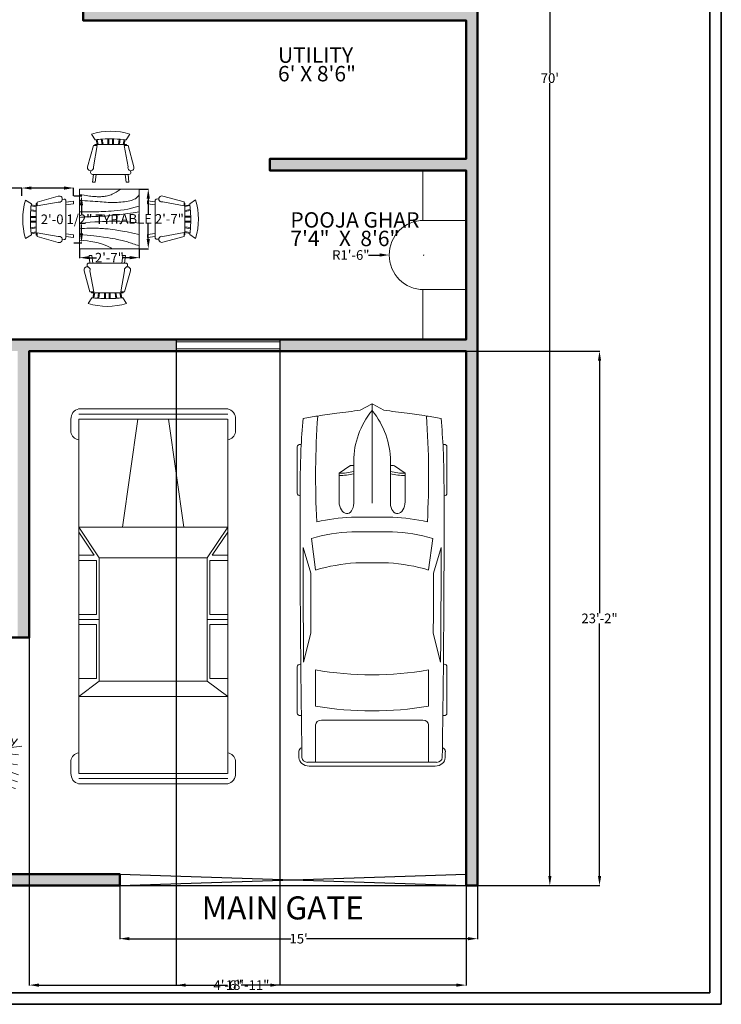
# Model space of a CAD drawing. Units: inches. Extents: x -60 to 743, y -483 to 510.
# Tile 4 of 7: x 378 to 743, y -483 to 29. Entities that reach past the tile are written whole.
import ezdxf

# ---------------------------------------------------------------- set-up
doc = ezdxf.new("R2010")
doc.units = ezdxf.units.IN
doc.header["$MEASUREMENT"] = 0
for name, color, linetype, lineweight in [('A-ANNO-DIMS', 2, 'Continuous', 18), ('A-ANNO-TEXT', 7, 'Continuous', 25), ('A-ANNO-TTLB', 7, 'Continuous', 35), ('A-AREA-IDEN', 7, 'Continuous', 25), ('A-WALL-PATT', 30, 'Continuous', 13), ('CARS', 131, 'Continuous', 13), ('FURNITURE', 40, 'Continuous', 18), ('GATE', 150, 'Continuous', 25), ('TREES', 80, 'Continuous', 13), ('WALL BOUNDRY', 10, 'Continuous', 50), ('WINDOW', 200, 'Continuous', 18)]:
    doc.layers.add(name, color=color, linetype=linetype, lineweight=lineweight)
doc.styles.get("Standard").update_dxf_attribs({"font": 'arial.ttf'})
doc.dimstyles.get("Standard").update_dxf_attribs({"dimtxt": 5, "dimasz": 5, "dimexe": 0.18, "dimexo": 0.0625, "dimgap": 0.09, "dimtad": 0, "dimtih": 1, "dimtoh": 1, "dimdec": 1, "dimzin": 0, "dimdsep": 46, "dimlunit": 4, "dimtxsty": 'Standard', "dimcen": 0.09, "dimadec": 0, "dimazin": 0, "dimtfac": 1, "dimtdec": 1, "dimtofl": 0, "dimtmove": 0, "dimatfit": 3, "dimfxl": 1, "dimtolj": 1, "dimtzin": 0, "dimarcsym": 0})

# ---------------------------------------------------------------- blocks, each defined once
blk = doc.blocks.new('Chair - Rocking')
for p, q in [((-8, -4.5), (-10, -1.5)), ((-7.5, -4.5), (-7, -7)), ((-6.5, -7), (-7.02225, -4.43)), ((-4.5, -7), (-4.96674, -4.19951)), ((-4, -7), (-4.40532, -4.16272)), ((-1.5, -4.05012), (-1.5, -7)), ((-1, -7), (-1, -4.05012)), ((1, -7), (1, -4.04655)), ((1.5, -4.05012), (1.5, -7)), ((4, -7), (4.40187, -4.18694)), ((4.5, -7), (4.96761, -4.19437)), ((6.5, -7), (7, -4.4057)), ((7.5, -4.5), (7, -7)), ((8, -4.5), (10, -1.5)), ((-9, -7.5), (-12, -18.49999)), ((-7, -7.5), (-9, -7.5)), ((-9, -18.49999), (-7, -7.5)), ((-8.23428, -6.99939), (-8.3093, -7.47958)), ((-8.23041, -7), (8.23915, -7)), ((7, -7.5), (9, -7.5)), ((9, -18.49999), (7, -7.5)), ((8.31071, -7.48854), (8.23449, -7.00073)), ((9, -7.5), (12, -18.49999)), ((-10.36644, -20.64523), (-10.5, -21.49999)), ((-9, -22.49999), (-9.5, -26.49999)), ((0, -22.49999), (-9.5, -22.49999)), ((-8, -26.49999), (-7.5, -22.49999)), ((0, -22.49999), (9.5, -22.49999)), ((8, -26.49999), (7.5, -22.49999)), ((9, -22.49999), (9.5, -26.49999)), ((10.5, -21.49999), (10.3575, -20.58798)), ((-9.5, -26.49999), (-8, -26.49999)), ((9.5, -26.49999), (8, -26.49999))]:
    blk.add_line(p, q)
for centre, radius, start, end in [((0, -34.08333), 34.08333, 72.93847, 107.0615), ((0, -68.25004), 64.25, 93.92211, 97.15267), ((0, -68.25004), 64.25, 82.84733, 93.92211), ((-10.5, -18.99999), 1.58114, 161.5651, 18.43495), ((10.5, -18.99999), 1.58114, 161.5651, 18.43495), ((-9.5, -21.49999), 1, 180, 270), ((9.5, -21.49999), 1, 270, 0)]:
    blk.add_arc(centre, radius, start, end)
blk = doc.blocks.new('Table - Square Woodgrain 42 x 42 in.')
blk.add_line((0, -42), (42, -42))
for points in [[(0, -4), (1.704, -4.2172), (3.2358, -4.4188), (4.615, -4.604), (5.8615, -4.7721), (6.9951, -4.9224), (8.0357, -5.0541), (9.0031, -5.1667), (9.9171, -5.2594), (10.7951, -5.3316), (11.6445, -5.3836), (12.4702, -5.4157), (13.277, -5.4283), (14.0698, -5.4217), (14.8535, -5.3964), (15.6331, -5.3526), (16.4133, -5.2908), (17.1986, -5.2103), (17.9913, -5.1062), (18.793, -4.9727), (19.6056, -4.8038), (20.4307, -4.5937), (21.2701, -4.3365), (22.1256, -4.0262), (22.9989, -3.6571), (23.888, -3.2272), (24.7756, -2.7516), (25.6408, -2.2491), (26.4624, -1.7387), (27.2195, -1.2395), (27.891, -0.7703), (28.456, -0.3501), (28.8934, 0.002)], [(0, -42), (0, 0), (42, 0), (42, -42)], [(0, -8), (1.8203, -8.1001), (3.6741, -8.2149), (5.5411, -8.3408), (7.4011, -8.4741), (9.2339, -8.6112), (11.0193, -8.7484), (12.7371, -8.8821), (14.3671, -9.0086), (15.8954, -9.1246), (17.3337, -9.2278), (18.6997, -9.3159), (20.0116, -9.387), (21.2871, -9.4389), (22.5442, -9.4696), (23.8008, -9.477), (25.0749, -9.459), (26.3791, -9.4137), (27.7049, -9.3403), (29.0383, -9.2382), (30.3655, -9.1068), (31.6728, -8.9455), (32.9461, -8.7535), (34.1717, -8.5304), (35.3358, -8.2756), (36.4268, -7.9863), (37.443, -7.6521), (38.3849, -7.2603), (39.253, -6.7986), (40.048, -6.2542), (40.7705, -5.6147), (41.421, -4.8674), (42, -4)], [(42, -12), (39.1784, -12.8621), (36.4519, -13.5654), (33.8246, -14.1294), (31.3004, -14.5731), (28.8832, -14.9161), (26.577, -15.1775), (24.3858, -15.3768), (22.3136, -15.5332), (20.3622, -15.6632), (18.5254, -15.7718), (16.7947, -15.8612), (15.1618, -15.9338), (13.6183, -15.9916), (12.1558, -16.0369), (10.7659, -16.0718), (9.4403, -16.0987), (8.1703, -16.1191), (6.9461, -16.1325), (5.7577, -16.1377), (4.595, -16.1335), (3.4479, -16.1188), (2.3064, -16.0924), (1.1604, -16.0532), (0, -16)], [(42, -16), (37.6529, -16.7365), (33.8802, -17.329), (30.6179, -17.7961), (27.8015, -18.1561), (25.3668, -18.4275), (23.2497, -18.6288), (21.3859, -18.7785), (19.7111, -18.8949), (18.1693, -18.9939), (16.7375, -19.0795), (15.401, -19.1534), (14.1449, -19.217), (12.9544, -19.2717), (11.8148, -19.3191), (10.7113, -19.3606), (9.6291, -19.3976), (8.5534, -19.4323), (7.47, -19.4689), (6.3643, -19.5122), (5.222, -19.5672), (4.0288, -19.6386), (2.7703, -19.7313), (1.4321, -19.8501), (0, -20)], [(0, -24), (3.9243, -23.6805), (7.4766, -23.4138), (10.6891, -23.1954), (13.5943, -23.0205), (16.2247, -22.8847), (18.6125, -22.7832), (20.7903, -22.7116), (22.7903, -22.6651), (24.6563, -22.642), (26.4764, -22.6507), (28.35, -22.7024), (30.3766, -22.8084), (32.6555, -22.98), (35.2861, -23.2283), (38.3678, -23.5645), (42, -24)], [(42, -32), (37.392, -31.017), (33.4585, -30.2231), (30.1291, -29.5949), (27.3334, -29.109), (25.0009, -28.742), (23.0612, -28.4707), (21.4439, -28.2716), (20.0786, -28.1215), (18.8998, -28.0002), (17.8609, -27.9014), (16.9206, -27.8219), (16.0371, -27.7588), (15.1691, -27.709), (14.2748, -27.6693), (13.3128, -27.6368), (12.2415, -27.6083), (11.0295, -27.5824), (9.6867, -27.5643), (8.233, -27.5608), (6.6884, -27.5787), (5.0728, -27.6248), (3.4062, -27.7058), (1.7086, -27.8286), (0, -28)], [(0, -32), (5.4026, -32.5358), (9.9494, -33.019), (13.7424, -33.4553), (16.8834, -33.8505), (19.4743, -34.2106), (21.6171, -34.5413), (23.4136, -34.8486), (24.9657, -35.1382), (26.3614, -35.4156), (27.6332, -35.6841), (28.7995, -35.9467), (29.8788, -36.2064), (30.8897, -36.4661), (31.8507, -36.7288), (32.7802, -36.9973), (33.6968, -37.2747), (34.6175, -37.5635), (35.5531, -37.8651), (36.5128, -38.1805), (37.506, -38.5108), (38.5421, -38.8568), (39.6302, -39.2197), (40.7797, -39.6004), (42, -40)], [(0, -36), (3.0098, -36.2857), (5.5354, -36.5643), (7.6368, -36.8359), (9.374, -37.1009), (10.807, -37.3597), (11.9957, -37.6126), (13.0002, -37.8599), (13.8804, -38.102), (14.6874, -38.3393), (15.4365, -38.5729), (16.1338, -38.8041), (16.7858, -39.0341), (17.3987, -39.264), (17.9787, -39.4952), (18.5322, -39.7288), (19.0655, -39.9662), (19.5832, -40.2081), (20.0842, -40.4544), (20.5657, -40.7046), (21.0249, -40.9581), (21.459, -41.2144), (21.8653, -41.4731), (22.2409, -41.7335), (22.5831, -41.9951)]]:
    blk.add_lwpolyline(points)
blk = doc.blocks.new('*U19')
for p, q in [((536, 950), (536, 936)), ((1182, 988), (568, 988)), ((1214, 950), (1214, 950)), ((2235, 810), (1899, 912)), ((3440, 942), (3440, 950)), ((3472, 988), (4087, 988)), ((4119, 950), (4119, 934)), ((1779, 801), (2195, 746)), ((3412, 904), (3030, 807)), ((4736, -851), (4736, 851)), ((4785, -832), (4785, 832)), ((3516, 746), (3994, 746)), ((4179, 670), (4179, -670)), ((4736, 746), (4242, 746)), ((820, 295), (918, 436)), ((918, 436), (1294, 436)), ((816, 241), (816, 283)), ((1496, -274), (1496, 274)), ((1690, -267), (1690, 267)), ((4736, -267), (4736, 267)), ((83, 156), (3, 10)), ((756, 241), (1313, 241)), ((2102, 216), (2102, -216)), ((0, 0), (1313, 0)), ((3, -10), (83, -156)), ((756, -241), (1313, -241)), ((816, -241), (816, -283)), ((820, -295), (918, -436)), ((918, -436), (1294, -436)), ((2195, -746), (1779, -801)), ((3994, -746), (3516, -746)), ((4242, -746), (4736, -746)), ((2235, -810), (1899, -912)), ((3412, -904), (3030, -807)), ((536, -950), (536, -936)), ((1182, -988), (568, -988)), ((1214, -950), (1214, -950)), ((3440, -942), (3440, -950)), ((3472, -988), (4087, -988)), ((4119, -950), (4119, -934))]:
    blk.add_line(p, q)
for centre, major_axis, ratio, start_param, end_param in [((6757, -699), (0, 7958), 0.842304, 1.367076, 1.39176), ((1046, -12468), (0, 13417), 0.842304, 0.00281, 0.075598), ((568, 950), (0, -37.6), 0.842304, 3.141593, 4.712389), ((1638, -268113), (0, 269063), 0.842304, -0.013397, 0.002797), ((1182, 950), (0, 37.6), 0.842304, -1.570796, 0), ((1638, -268113), (0, -269025), 0.842304, 3.133765, 3.140441), ((3472, 950), (0, -37.6), 0.842304, 3.141593, 4.712389), ((4087, 950), (0, 37.6), 0.842304, -1.570796, 0), ((4588, 910), (0, 56.4), 0.842304, -0.013017, 1.249894), ((1638, -268131), (0, 269121), 0.842304, -0.013397, -0.013017), ((4673, 851), (0, -75.2), 0.842304, 1.570796, 3.128196), ((4673, 832), (0, -133), 0.842304, 1.570796, 3.128196), ((3436, 137), (0, 2077), 0.842304, 1.245306, 1.50788), ((2433, -93125), (0, -93935), 0.842304, 3.134049, 3.144098), ((6583, -699), (0, -7755), 0.842304, 4.528606, 4.561838), ((952, -15087), (0, -15833), 0.842304, 3.096046, 3.200911), ((3414, 137), (0, -2280), 0.842304, 4.449482, 4.652344), ((3800, 71), (0, -2021), 0.842304, 4.372215, 4.640744), ((434, 0), (0, 3734), 0.842304, 4.511394, 4.913384), ((912, 0), (0, 3734), 0.842304, 4.511394, 4.913384), ((4242, 670), (0, 75.2), 0.842304, 0, 1.570796), ((-5194, 1331), (0, -6374), 0.842304, 1.385369, 1.434372), ((331, 432), (0, 696), 0.842304, 4.435146, 4.718221), ((361, 432), (0, 696), 0.842304, 4.435146, 4.718221), ((1290, 339), (161, -9), 0.603834, -1.395552, 1.581315), ((832, 283), (0, 18.8), 0.842304, 0.879714, 1.570796), ((756, -1185), (0, 1427), 0.842304, 0, 0.590319), ((16, 0), (0, -18.8), 0.842304, 4.131459, 5.293319), ((756, 1185), (0, 1427), 0.842304, 2.551274, 3.141593), ((-5194, -1331), (0, 6374), 0.842304, -1.434372, -1.385369), ((331, -432), (0, -696), 0.842304, 1.564964, 1.848039), ((361, -432), (0, -696), 0.842304, 1.564964, 1.848039), ((3800, -71), (0, -2021), 0.842304, -1.499151, -1.230623), ((832, -283), (0, -18.8), 0.842304, 4.712389, 5.403472), ((3414, -137), (0, -2280), 0.842304, -1.510751, -1.307889), ((3436, -137), (0, -2077), 0.842304, -1.50788, -1.245306), ((6583, 699), (0, 7755), 0.842304, 1.721348, 1.754579), ((6757, 699), (0, 7958), 0.842304, 1.749832, 1.774517), ((952, 15087), (0, -15833), 0.842304, -0.059319, 0.045547), ((4242, -670), (0, -75.2), 0.842304, 4.712389, 6.283185), ((1638, 268113), (0, -269025), 0.842304, 0.001152, 0.007828), ((2433, 93125), (0, -93935), 0.842304, -0.002505, 0.007544), ((4673, -851), (0, 75.2), 0.842304, 3.15499, 4.712389), ((4673, -832), (0, -133), 0.842304, 0.013397, 1.570796), ((1046, 12468), (0, -13417), 0.842304, -0.075598, -0.00281), ((568, -950), (0, 37.6), 0.842304, 1.570796, 3.141593), ((1638, 268113), (0, 269063), 0.842304, 3.138796, 3.15499), ((1182, -950), (0, -37.6), 0.842304, 0, 1.570796), ((3472, -950), (0, -37.6), 0.842304, -1.570796, 0), ((4087, -950), (0, 37.6), 0.842304, 3.141593, 4.712389), ((4588, -910), (0, -56.4), 0.842304, -1.249894, 0.013017), ((1638, 268131), (0, 269121), 0.842304, 3.15461, 3.15499)]:
    blk.add_ellipse(centre, major_axis=major_axis, ratio=ratio, start_param=start_param, end_param=end_param)
at = {"extrusion": (0, 0, -1)}
blk.add_ellipse((1290, -339), major_axis=(161, 9), ratio=0.603834, start_param=-1.395552, end_param=1.581315, dxfattribs=at)
blk = doc.blocks.new('*U18')
for p, q in [((138, 1075), (308, 1075)), ((4818, 1075), (4649, 1075)), ((3, -10), (3, 974)), ((70, -10), (70, 973)), ((138, 973), (410, 973)), ((138, -10), (138, 971)), ((410, 973), (4581, 973)), ((1563, -10), (1563, 973)), ((1563, 973), (1969, 702)), ((1630, 973), (1936, 769)), ((1936, 769), (1936, 973)), ((2003, 973), (2003, 736)), ((2716, 736), (2716, 973)), ((2783, 702), (2783, 973)), ((2851, 973), (2851, 736)), ((3563, 736), (3563, 973)), ((3597, 702), (3801, 973)), ((3801, -10), (3801, 973)), ((4818, 973), (4547, 973)), ((4818, -10), (4818, 971)), ((4886, -10), (4886, 973)), ((4954, -10), (4954, 974)), ((1969, 702), (3597, 702)), ((1969, -10), (1969, 702)), ((2003, 736), (2716, 736)), ((2851, 736), (3563, 736)), ((3597, -10), (3597, 702)), ((138, 193), (1563, 396)), ((3, -11), (3, -995)), ((70, -10), (70, -994)), ((138, -11), (138, -992)), ((1563, -10), (1563, -994)), ((1969, -10), (1969, -723)), ((3597, -10), (3597, -723)), ((3801, -10), (3801, -994)), ((4818, -11), (4818, -992)), ((4886, -10), (4886, -994)), ((4954, -11), (4954, -995)), ((138, -214), (1563, -417)), ((1563, -994), (1969, -723)), ((1969, -723), (3597, -723)), ((2003, -994), (2003, -757)), ((2003, -757), (2716, -757)), ((2716, -757), (2716, -994)), ((2783, -723), (2783, -994)), ((2851, -757), (3563, -757)), ((2851, -994), (2851, -757)), ((3563, -757), (3563, -994)), ((3597, -723), (3801, -994)), ((1630, -994), (1936, -790)), ((1936, -790), (1936, -994)), ((138, -994), (410, -994)), ((410, -994), (4581, -994)), ((4818, -994), (4547, -994)), ((138, -1096), (308, -1096)), ((4818, -1096), (4649, -1096))]:
    blk.add_line(p, q)
for centre, radius, start, end in [((128, 946), 129, 85.6455, 168.0943), ((291, 956), 120, 8.1301, 81.87), ((4665, 956), 120, 98.13, 171.8699), ((4828, 946), 129, 11.9057, 94.3545), ((128, -967), 129, 191.9057, 274.3545), ((291, -977), 120, 278.13, 351.8699), ((4665, -977), 120, 188.1301, 261.87), ((4828, -967), 129, 265.6455, 348.0943)]:
    blk.add_arc(centre, radius, start, end)
blk = doc.blocks.new('*U21')
for p, q in [((-258.7244, 1362.456), (-332.3336, 1421.4348)), ((0, 0), (-266.7, 1447.8)), ((-231.1146, 1315.2628), (-166.7002, 1421.4348)), ((-221.9198, 1197.3052), (-433.5526, 1338.8594)), ((-194.31, 1102.9442), (-65.4812, 1256.284)), ((-148.3106, 914.1968), (118.5418, 1220.9018)), ((-185.1152, 1008.5578), (-553.1612, 1185.4942)), ((-129.8956, 701.8528), (265.7602, 1185.4942)), ((-93.091, 489.5342), (-700.3796, 902.3858)), ((-129.8956, 713.6638), (-626.7704, 1032.1544)), ((-74.7014, 418.7444), (219.7608, 961.39)), ((685.8, 228.6), (1219.2, 914.4)), ((689.0258, 230.0224), (790.2448, 914.1968)), ((983.4626, 867.0036), (1066.2666, 725.4494)), ((1121.4862, 925.9824), (1149.0706, 831.6214)), ((-1234.059, 536.7274), (-1252.4486, 737.2604)), ((-1105.2302, 725.4494), (-1077.6458, 395.1732)), ((-902.8176, 713.6638), (-617.5756, 100.2538)), ((412.9786, 147.447), (587.8068, 796.2392)), ((560.197, 182.8292), (698.2206, 819.8358)), ((808.6344, 784.4282), (827.0494, 418.7444)), ((891.4384, 831.6214), (946.658, 572.1096)), ((1112.2914, 760.8316), (1296.3144, 784.4282)), ((-800.1, 114.3), (-1333.5, 647.7)), ((-976.4268, 666.4706), (-884.4026, 194.6402)), ((-369.1382, 53.086), (-783.1836, 642.874)), ((-617.5756, 607.4918), (-74.7014, 347.98)), ((-28.6766, 171.0436), (228.9556, 678.2816)), ((100.1268, 41.275), (284.1498, 619.2774)), ((256.5654, 88.4682), (449.7832, 666.4706)), ((1029.462, 654.685), (1241.0948, 631.0884)), ((-1206.4492, 501.3198), (-1418.082, 465.9376)), ((-1031.621, 347.98), (-1399.667, 277.1902)), ((-525.5514, 347.98), (-28.6766, 123.8504)), ((845.439, 418.7444), (1241.0948, 277.1902)), ((919.0482, 501.3198), (1222.6798, 454.152)), ((0, 0), (685.8, 228.6)), ((615.4166, 194.6402), (1185.8752, 41.275)), ((753.4148, 312.5978), (1222.6798, 159.2326)), ((-847.598, 159.2326), (-1326.0578, 135.636)), ((-718.7946, 88.4682), (-1215.644, -147.447)), ((-543.9664, 76.6572), (-967.2066, -206.4512)), ((0, 0), (-800.1, 114.3)), ((-405.9428, 53.086), (-764.794, -241.8334)), ((0, 0), (-571.5, -495.3)), ((-166.7002, 29.4894), (-543.9664, -206.4512)), ((0, 0), (457.2, -571.5)), ((164.5412, 41.275), (661.416, -218.2368)), ((284.1498, 88.4682), (781.0246, -147.447)), ((458.978, 147.447), (891.4384, -88.4682)), ((-166.7002, -147.447), (-507.1618, -253.619)), ((-120.7008, -88.4682), (-93.091, -371.5766)), ((63.3222, -76.6826), (-37.8714, -513.1308)), ((44.9326, -64.897), (615.4166, -241.8334)), ((127.7366, -159.258), (54.1274, -654.685)), ((-387.5278, -324.4088), (-764.794, -324.4088)), ((-341.5284, -289.0012), (-221.9198, -831.6214)), ((-240.3094, -218.2368), (-157.5054, -595.7062)), ((228.9556, -289.0012), (90.932, -914.1968)), ((192.151, -230.0224), (817.8292, -371.5766)), ((-442.7474, -383.3876), (-1086.8406, -477.7486)), ((-571.5, -495.3), (-952.5, -1143)), ((-525.5514, -465.963), (-451.9422, -1126.5408)), ((-433.5526, -383.3876), (-323.1134, -1020.3688)), ((357.759, -430.5554), (164.5412, -1020.3688)), ((311.7596, -383.3876), (937.4378, -477.7486)), ((412.9786, -501.3452), (919.0482, -583.9206)), ((-617.5756, -548.5384), (-1077.6458, -560.324)), ((-681.9646, -666.496), (-1022.4262, -654.685)), ((-635.9652, -607.5172), (-580.771, -1150.1374)), ((458.978, -572.1096), (210.5406, -1161.923)), ((457.2, -571.5), (685.8, -1333.5)), ((468.1982, -572.1096), (1029.462, -737.2604)), ((486.5878, -642.8994), (983.4626, -843.4324)), ((-718.7946, -737.2604), (-1086.8406, -796.2392)), ((-737.1842, -784.4536), (-709.5744, -1114.7298)), ((514.1976, -772.6426), (403.7838, -1138.3264)), ((541.8074, -831.6214), (992.6574, -1032.1544)), ((-783.1836, -867.029), (-1077.6458, -902.4112)), ((-875.2078, -1008.5832), (-1040.8412, -1079.3476)), ((-829.2084, -937.7934), (-810.7934, -1126.5408)), ((578.612, -961.39), (495.7826, -1232.7128)), ((578.612, -973.1756), (873.0488, -1138.3264)), ((624.6114, -1161.923), (587.8068, -1291.6916)), ((624.6114, -1102.9442), (781.0246, -1209.1162)), ((679.8056, -1268.095), (716.6102, -1291.6916))]:
    blk.add_line(p, q)
blk = doc.blocks.new('*D23')
at = {"layer": 'A-ANNO-DIMS', "color": 0, "lineweight": -2, "transparency": 16777216}
for p, q in [((616.21, 418.42), (653.91, 418.42)), ((653.73, 413.42), (653.73, 1.06)), ((653.73, -416.58), (653.73, -4.22)), ((616.21, -421.58), (653.91, -421.58))]:
    blk.add_line(p, q, dxfattribs=at)
at = {"layer": 'A-ANNO-DIMS', "color": 0, "transparency": 16777216}
for points in [[(652.9, 413.42), (654.56, 413.42), (653.73, 418.42)], [(652.9, -416.58), (654.56, -416.58), (653.73, -421.58)]]:
    blk.add_solid(points, dxfattribs=at)
at = {"layer": 'Defpoints', "color": 0, "transparency": 16777216}
for p in [(616.15, 418.42), (616.15, -421.58), (653.73, -421.58)]:
    blk.add_point(p, dxfattribs=at)
at = {"layer": 'A-ANNO-DIMS', "color": 0, "transparency": 16777216, "insert": (653.73, -1.58), "char_height": 5, "attachment_point": 5}
blk.add_mtext("\\A1;70'", dxfattribs=at)
blk = doc.blocks.new('*D24')
at = {"layer": 'A-ANNO-DIMS', "color": 0, "lineweight": -2, "transparency": 16777216}
for p, q in [((430.15, -421.64), (430.15, -449.36)), ((616.15, -421.64), (616.15, -449.36)), ((435.15, -449.18), (519.05, -449.18)), ((611.15, -449.18), (527.24, -449.18))]:
    blk.add_line(p, q, dxfattribs=at)
at = {"layer": 'A-ANNO-DIMS', "color": 0, "transparency": 16777216}
for points in [[(435.15, -448.34), (435.15, -450.01), (430.15, -449.18)], [(611.15, -448.34), (611.15, -450.01), (616.15, -449.18)]]:
    blk.add_solid(points, dxfattribs=at)
at = {"layer": 'Defpoints', "color": 0, "transparency": 16777216}
for p in [(430.15, -421.58), (616.15, -421.58), (616.15, -449.18)]:
    blk.add_point(p, dxfattribs=at)
at = {"layer": 'A-ANNO-DIMS', "color": 0, "transparency": 16777216, "insert": (523.15, -449.18), "char_height": 5, "attachment_point": 5}
blk.add_mtext("\\A1;15'", dxfattribs=at)
blk = doc.blocks.new('*D34')
at = {"layer": 'A-ANNO-DIMS', "color": 0, "lineweight": -2, "transparency": 16777216}
for p, q in [((379.23, -58.74), (374.23, -58.74)), ((379.23, -62.73), (379.23, -58.56)), ((401.23, -58.74), (384.23, -58.74)), ((406.23, -62.73), (406.23, -58.56))]:
    blk.add_line(p, q, dxfattribs=at)
at = {"layer": 'A-ANNO-DIMS', "color": 0, "transparency": 16777216}
for points in [[(384.23, -57.91), (384.23, -59.58), (379.23, -58.74)], [(401.23, -57.91), (401.23, -59.58), (406.23, -58.74)]]:
    blk.add_solid(points, dxfattribs=at)
at = {"layer": 'Defpoints', "color": 0, "transparency": 16777216}
for p in [(379.23, -58.74), (379.23, -62.79), (406.23, -62.79)]:
    blk.add_point(p, dxfattribs=at)
at = {"layer": 'A-ANNO-DIMS', "color": 0, "transparency": 16777216, "insert": (343.12, -58.74), "char_height": 5, "attachment_point": 5}
blk.add_mtext('\\A1;ROCKER 2\'-3" TYP.', dxfattribs=at)
blk = doc.blocks.new('*D35')
at = {"layer": 'A-ANNO-DIMS', "color": 0, "lineweight": -2, "transparency": 16777216}
for p, q in [((406.29, -62.79), (410.46, -62.79)), ((410.28, -67.79), (410.28, -72.33)), ((410.28, -82.23), (410.28, -77.68)), ((406.29, -87.23), (410.46, -87.23))]:
    blk.add_line(p, q, dxfattribs=at)
at = {"layer": 'A-ANNO-DIMS', "color": 0, "transparency": 16777216}
for points in [[(409.44, -67.79), (411.11, -67.79), (410.28, -62.79)], [(409.44, -82.23), (411.11, -82.23), (410.28, -87.23)]]:
    blk.add_solid(points, dxfattribs=at)
at = {"layer": 'Defpoints', "color": 0, "transparency": 16777216}
for p in [(406.23, -62.79), (410.28, -62.79), (406.23, -87.23)]:
    blk.add_point(p, dxfattribs=at)
at = {"layer": 'A-ANNO-DIMS', "color": 0, "transparency": 16777216, "insert": (410.28, -75.01), "char_height": 5, "attachment_point": 5}
blk.add_mtext('\\A1;2\'-0 1/2" TYP.', dxfattribs=at)
blk = doc.blocks.new('*D64')
at = {"layer": 'A-ANNO-DIMS', "color": 0, "lineweight": -2, "transparency": 16777216}
for p, q in [((440.41, -59.25), (445.19, -59.25)), ((445.01, -64.25), (445.01, -72.18)), ((445.01, -85.31), (445.01, -77.38)), ((440.41, -90.31), (445.19, -90.31))]:
    blk.add_line(p, q, dxfattribs=at)
at = {"layer": 'A-ANNO-DIMS', "color": 0, "transparency": 16777216}
for points in [[(444.18, -64.25), (445.84, -64.25), (445.01, -59.25)], [(444.18, -85.31), (445.84, -85.31), (445.01, -90.31)]]:
    blk.add_solid(points, dxfattribs=at)
at = {"layer": 'Defpoints', "color": 0, "transparency": 16777216}
for p in [(440.35, -59.25), (445.01, -59.25), (440.35, -90.31)]:
    blk.add_point(p, dxfattribs=at)
at = {"layer": 'A-ANNO-DIMS', "color": 0, "transparency": 16777216, "insert": (445.01, -74.78), "char_height": 5, "attachment_point": 5}
blk.add_mtext('\\A1;TABLE 2\'-7"', dxfattribs=at)
blk = doc.blocks.new('*D65')
at = {"layer": 'A-ANNO-DIMS', "color": 0, "lineweight": -2, "transparency": 16777216}
for p, q in [((409.3, -90.37), (409.3, -95.15)), ((440.35, -90.37), (440.35, -95.15)), ((414.3, -94.97), (418.05, -94.97)), ((435.35, -94.97), (431.6, -94.97))]:
    blk.add_line(p, q, dxfattribs=at)
at = {"layer": 'A-ANNO-DIMS', "color": 0, "transparency": 16777216}
for points in [[(414.3, -94.13), (414.3, -95.8), (409.3, -94.97)], [(435.35, -94.13), (435.35, -95.8), (440.35, -94.97)]]:
    blk.add_solid(points, dxfattribs=at)
at = {"layer": 'Defpoints', "color": 0, "transparency": 16777216}
for p in [(409.3, -90.31), (440.35, -90.31), (440.35, -94.97)]:
    blk.add_point(p, dxfattribs=at)
at = {"layer": 'A-ANNO-DIMS', "color": 0, "transparency": 16777216, "insert": (424.82, -94.97), "char_height": 5, "attachment_point": 5}
blk.add_mtext('\\A1;2\'-7"', dxfattribs=at)
blk = doc.blocks.new('*D70')
at = {"layer": 'A-ANNO-DIMS', "color": 0, "lineweight": -2, "transparency": 16777216}
for p, q in [((610.21, -143.58), (679.73, -143.58)), ((679.55, -148.58), (679.55, -279.93)), ((679.55, -416.58), (679.55, -285.22)), ((616.21, -421.58), (679.73, -421.58))]:
    blk.add_line(p, q, dxfattribs=at)
at = {"layer": 'A-ANNO-DIMS', "color": 0, "transparency": 16777216}
for points in [[(678.72, -148.58), (680.39, -148.58), (679.55, -143.58)], [(678.72, -416.58), (680.39, -416.58), (679.55, -421.58)]]:
    blk.add_solid(points, dxfattribs=at)
at = {"layer": 'Defpoints', "color": 0, "transparency": 16777216}
for p in [(610.15, -143.58), (679.55, -143.58), (616.15, -421.58)]:
    blk.add_point(p, dxfattribs=at)
at = {"layer": 'A-ANNO-DIMS', "color": 0, "transparency": 16777216, "insert": (679.55, -282.58), "char_height": 5, "attachment_point": 5}
blk.add_mtext('\\A1;23\'-2"', dxfattribs=at)
blk = doc.blocks.new('*D71')
at = {"layer": 'A-ANNO-DIMS', "color": 0, "lineweight": -2, "transparency": 16777216}
for p, q in [((383.15, -292.64), (383.15, -473.51)), ((610.15, -415.64), (610.15, -473.51)), ((388.15, -473.33), (486.26, -473.33)), ((605.15, -473.33), (507.03, -473.33))]:
    blk.add_line(p, q, dxfattribs=at)
at = {"layer": 'A-ANNO-DIMS', "color": 0, "transparency": 16777216}
for points in [[(388.15, -472.5), (388.15, -474.17), (383.15, -473.33)], [(605.15, -472.5), (605.15, -474.17), (610.15, -473.33)]]:
    blk.add_solid(points, dxfattribs=at)
at = {"layer": 'Defpoints', "color": 0, "transparency": 16777216}
for p in [(383.15, -292.58), (610.15, -415.58), (610.15, -473.33)]:
    blk.add_point(p, dxfattribs=at)
at = {"layer": 'A-ANNO-DIMS', "color": 0, "transparency": 16777216, "insert": (496.65, -473.33), "char_height": 5, "attachment_point": 5}
blk.add_mtext('\\A1;18\'-11"', dxfattribs=at)
blk = doc.blocks.new('*D83')
at = {"layer": 'A-ANNO-DIMS', "color": 0, "lineweight": -2, "transparency": 16777216}
for p, q in [((459.53, -137.64), (459.53, -473.51)), ((513.39, -137.64), (513.39, -473.51)), ((464.53, -473.33), (479.62, -473.33)), ((508.39, -473.33), (493.3, -473.33))]:
    blk.add_line(p, q, dxfattribs=at)
at = {"layer": 'A-ANNO-DIMS', "color": 0, "transparency": 16777216}
for points in [[(464.53, -472.5), (464.53, -474.17), (459.53, -473.33)], [(508.39, -472.5), (508.39, -474.17), (513.39, -473.33)]]:
    blk.add_solid(points, dxfattribs=at)
at = {"layer": 'Defpoints', "color": 0, "transparency": 16777216}
for p in [(459.53, -137.58), (513.39, -137.58), (513.39, -473.33)]:
    blk.add_point(p, dxfattribs=at)
at = {"layer": 'A-ANNO-DIMS', "color": 0, "transparency": 16777216, "insert": (486.46, -473.33), "char_height": 5, "attachment_point": 5}
blk.add_mtext('\\A1;4\'-6"', dxfattribs=at)
blk = doc.blocks.new('*D84')
at = {"layer": 'A-ANNO-DIMS', "color": 0, "lineweight": -2, "transparency": 16777216}
for p, q in [((559.42, -93.58), (565.22, -93.58)), ((588.13, -93.58), (588.31, -93.58)), ((588.22, -93.67), (588.22, -93.49))]:
    blk.add_line(p, q, dxfattribs=at)
at = {"layer": 'A-ANNO-DIMS', "color": 0, "transparency": 16777216}
blk.add_solid([(565.22, -92.74), (565.22, -94.41), (570.22, -93.58)], dxfattribs=at)
at = {"layer": 'Defpoints', "color": 0, "transparency": 16777216}
for p in [(570.22, -93.58), (588.22, -93.58)]:
    blk.add_point(p, dxfattribs=at)
at = {"layer": 'A-ANNO-DIMS', "color": 0, "transparency": 16777216, "insert": (550.29, -93.58), "char_height": 5, "attachment_point": 5}
blk.add_mtext('\\A1;R1\'-6"', dxfattribs=at)

msp = doc.modelspace()

# ---------------------------------------------------------------- hatches: boundary and pattern name
at = {"layer": 'A-WALL-PATT'}
h = msp.add_hatch(color=256, dxfattribs=at)
h.dxf.hatch_style = 1
h.paths.add_polyline_path([(412.35, 168.77), (415.89, 168.77), (415.89, 114.92), (412.35, 114.92)], flags=16)
h.paths.add_polyline_path([(87.81, -138.81), (87.81, -142.35), (48.31, -142.32), (48.31, -138.78)], flags=16)
h.paths.add_polyline_path([(459.53, -138.78), (513.39, -138.78), (513.39, -142.32), (459.53, -142.32)], flags=16)
h.paths.add_polyline_path([(164.84, -257.78), (218.7, -257.78), (218.7, -261.32), (164.84, -261.32)], flags=16)
h.paths.add_polyline_path([(417.15, 114.92), (415.89, 114.92), (415.89, 168.77), (417.15, 168.77), (417.15, 195.42), (411.15, 195.42), (411.15, 168.77), (412.35, 168.77), (412.35, 114.92), (411.15, 114.92), (411.15, 28.42), (610.15, 28.42), (610.15, -43.58), (508.15, -43.58), (508.15, -49.58), (610.15, -49.58), (610.15, -137.58), (513.39, -137.58), (513.39, -138.78), (459.53, -138.78), (459.53, -137.58), (359.15, -137.58), (359.15, -143.58), (377.15, -143.58), (377.15, -292.58), (383.15, -292.58), (383.15, -143.58), (459.53, -143.58), (459.53, -142.32), (513.39, -142.32), (513.39, -143.58), (610.15, -143.58), (610.15, -415.58), (610.15, -421.58), (616.15, -421.58), (616.15, 418.42), (13.15, 418.42), (13.15, -421.58), (19.15, -421.58), (430.15, -421.58), (430.15, -415.58), (19.15, -415.58), (19.15, -143.58), (48.31, -143.58), (48.31, -142.32), (87.81, -142.35), (87.81, -143.58), (117.15, -143.58), (117.15, -262.58), (164.84, -262.58), (164.84, -261.32), (218.7, -261.32), (218.7, -262.58), (273.15, -262.58), (273.15, -292.58), (279.15, -292.58), (279.15, -143.58), (297.15, -143.58), (297.15, -137.58), (273.15, -137.58), (273.15, -256.58), (218.7, -256.58), (218.7, -257.78), (164.84, -257.78), (164.84, -256.58), (123.15, -256.58), (123.15, -143.58), (225.15, -143.58), (225.15, -137.58), (87.81, -137.58), (87.81, -138.81), (48.31, -138.78), (48.31, -137.58), (19.15, -137.58), (19.15, 28.42), (187.15, 28.42), (187.15, 34.42), (19.15, 34.42), (19.15, 178.42), (273.15, 178.42), (273.15, 184.42), (19.15, 184.42), (19.15, 345.58), (195.14, 345.58), (195.14, 348.9), (19.15, 348.9), (19.15, 412.42), (267.15, 412.42), (267.15, 319.83), (273.15, 319.83), (273.15, 412.42), (411.15, 412.42), (411.15, 376.24), (417.15, 376.24), (417.15, 412.42), (610.15, 412.42), (610.15, 249.42), (411.15, 249.42), (411.15, 243.42), (610.15, 243.42), (610.15, 34.42), (417.15, 34.42)])
h = msp.add_hatch(color=256, dxfattribs=at)
h.dxf.hatch_style = 1
h.paths.add_polyline_path([(273.15, 265.98), (267.15, 265.98), (267.15, 232.42), (273.15, 232.42)])
h.paths.add_polyline_path([(417.15, 322.39), (411.15, 322.39), (411.15, 297.42), (417.15, 297.42)])
h.paths.add_polyline_path([(417.15, 195.42), (411.15, 195.42), (411.15, 168.77), (417.15, 168.77)])
h.paths.add_polyline_path([(459.53, -137.58), (359.15, -137.58), (359.15, -143.58), (377.15, -143.58), (377.15, -292.58), (383.15, -292.58), (383.15, -143.58), (459.53, -143.58)])
h.paths.add_polyline_path([(279.15, -143.58), (297.15, -143.58), (297.15, -137.58), (273.15, -137.58), (273.15, -256.58), (218.7, -256.58), (218.7, -262.58), (273.15, -262.58), (273.15, -292.58), (279.15, -292.58)])
h.paths.add_polyline_path([(123.15, -143.58), (225.15, -143.58), (225.15, -137.58), (87.81, -137.58), (87.81, -143.58), (117.15, -143.58), (117.15, -262.58), (164.84, -262.58), (164.84, -256.58), (123.15, -256.58)])

# ---------------------------------------------------------------- linework, layer by layer
at = {"layer": 'A-ANNO-TTLB'}
for points in [[(742.84, -483.31), (-60.19, -483.31), (-60.19, 510.12), (742.84, 510.12)], [(736.84, -477.31), (-54.19, -477.31), (-54.19, 504.12), (736.84, 504.12)]]:
    msp.add_lwpolyline(points, close=True, dxfattribs=at)
at = {"layer": 'FURNITURE'}
for points in [[(587.72, -49.58), (587.72, -75.58), (598.93, -75.58), (610.15, -75.58)], [(587.72, -137.58), (587.72, -111.58), (598.93, -111.58), (610.15, -111.58)]]:
    msp.add_lwpolyline(points, dxfattribs=at)
msp.add_arc((588.22, -93.58), 18, 90, 270, dxfattribs=at)
at = {"layer": 'GATE'}
for p, q in [((430.15, -415.58), (610.15, -421.58)), ((430.15, -421.58), (610.15, -415.58)), ((430.15, -421.58), (616.15, -421.58))]:
    msp.add_line(p, q, dxfattribs=at)
at = {"layer": 'WALL BOUNDRY'}
msp.add_lwpolyline([(610.15, -415.58), (610.15, -421.58), (616.15, -421.58), (616.15, 418.42), (13.15, 418.42), (13.15, -421.58), (19.15, -421.58), (430.15, -421.58), (430.15, -415.58), (19.15, -415.58), (19.15, -143.58), (117.15, -143.58), (117.15, -262.58), (273.15, -262.58), (273.15, -292.58), (279.15, -292.58), (377.15, -292.58), (383.15, -292.58), (383.15, -143.58), (610.15, -143.58)], close=True, dxfattribs=at)
msp.add_lwpolyline([(411.15, 195.42), (411.15, 28.42), (610.15, 28.42), (610.15, -43.58), (508.15, -43.58), (508.15, -49.58), (610.15, -49.58), (610.15, -137.58), (359.15, -137.58)], dxfattribs=at)
at = {"layer": 'WINDOW'}
for points in [[(513.39, -137.58), (513.39, -143.58), (459.53, -143.58), (459.53, -137.58)], [(513.39, -138.78), (513.39, -142.32), (459.53, -142.32), (459.53, -138.78)]]:
    msp.add_lwpolyline(points, close=True, dxfattribs=at)

# ---------------------------------------------------------------- block references
at = {"layer": 'CARS', "xscale": 0.0393700787401575, "yscale": 0.0393700787401575, "zscale": 0.0393700787401575, "rotation": 270}
for name, p in [('*U18', (447.98, -173.55)), ('*U19', (561.34, -170.99))]:
    msp.add_blockref(name, p, dxfattribs=at)
at = {"layer": 'FURNITURE'}
msp.add_blockref('Chair - Rocking', (425.49, -29.17), dxfattribs=at)
at = {"layer": 'FURNITURE', "xscale": 0.7394035319580894, "yscale": 0.7394035319580894, "zscale": 0.7394035319580894}
msp.add_blockref('Table - Square Woodgrain 42 x 42 in.', (409.3, -59.25), dxfattribs=at)
at = {"layer": 'FURNITURE'}
for p, rotation in [((379.73, -75.01), 90), ((471.08, -74.92), 270), ((423.72, -120.29), 180)]:
    msp.add_blockref('Chair - Rocking', p, dxfattribs=dict(at, rotation=rotation))
at = {"layer": 'TREES', "xscale": 0.0295751403229488, "yscale": 0.0295751403229488, "zscale": 0.0295751403229488}
msp.add_blockref('*U21', (340.92, -372.23), dxfattribs=at)

# ---------------------------------------------------------------- texts
at = {"layer": 'A-ANNO-TEXT'}
msp.add_text('MAIN GATE', height=12, dxfattribs=at).set_placement((472.77, -439.18))
at = {"layer": 'A-AREA-IDEN'}
for s, p in [('UTILITY', (512.42, 6.38)), ('6\' X 8\'6"', (512.42, -3.26)), ('POOJA GHAR', (518.88, -79.33)), ('7\'4"  X  8\'6"', (518.88, -88.96))]:
    msp.add_text(s, height=8, dxfattribs=at).set_placement(p)

# ---------------------------------------------------------------- dimensions: what is measured, and where the dimension line sits
at = {"layer": 'A-ANNO-DIMS'}
for base, p1, p2, override, picture, middle in [((653.73, -421.58), (616.15, 418.42), (616.15, -421.58), {"dimclrd": 0, "dimclre": 0, "dimclrt": 0}, '*D23', (653.73, -1.58)), ((679.55, -143.58), (616.15, -421.58), (610.15, -143.58), {"dimdec": 1, "dimlfac": 1, "dimrnd": 0, "dimzin": 1, "dimdsep": 46, "dimlunit": 4, "dimfrac": 2}, '*D70', (679.55, -282.58))]:
    dim = msp.add_linear_dim(base=base, p1=p1, p2=p2, angle=90, dimstyle='Standard', override=override, dxfattribs=at)
    dim.commit()
    dim.dimension.update_dxf_attribs({"geometry": picture, "text_midpoint": middle})
for base, p1, p2, angle, text, picture, middle in [((379.23, -58.74), (406.23, -62.79), (379.23, -62.79), 180, 'ROCKER <> TYP.', '*D34', (343.12, -58.74)), ((445.01, -59.25), (440.35, -90.31), (440.35, -59.25), 90, 'TABLE <>', '*D64', (445.01, -74.78)), ((410.28, -62.79), (406.23, -87.23), (406.23, -62.79), 90, '<> TYP.', '*D35', (410.28, -75.01))]:
    dim = msp.add_linear_dim(base=base, p1=p1, p2=p2, angle=angle, text=text, dimstyle='Standard', override={"dimdec": 1, "dimlfac": 1, "dimrnd": 0, "dimzin": 1, "dimdsep": 46, "dimlunit": 4, "dimfrac": 2}, dxfattribs=at)
    dim.commit()
    dim.dimension.update_dxf_attribs({"geometry": picture, "text_midpoint": middle})
for base, p1, p2, picture, middle in [((440.3517, -94.9682), (409.2968, -90.3097), (440.3517, -90.3097), '*D65', (424.8243, -94.9682)), ((513.39, -473.33), (459.53, -137.58), (513.39, -137.58), '*D83', (486.46, -473.33)), ((610.15, -473.33), (383.15, -292.58), (610.15, -415.58), '*D71', (496.65, -473.33))]:
    dim = msp.add_linear_dim(base=base, p1=p1, p2=p2, dimstyle='Standard', override={"dimdec": 1, "dimlfac": 1, "dimrnd": 0, "dimzin": 1, "dimdsep": 46, "dimlunit": 4, "dimfrac": 2}, dxfattribs=at)
    dim.commit()
    dim.dimension.update_dxf_attribs({"geometry": picture, "text_midpoint": middle})
dim = msp.add_radius_dim(center=(588.22, -93.58), mpoint=(570.22, -93.58), dimstyle='Standard', override={"dimdec": 1, "dimlfac": 1, "dimrnd": 0, "dimzin": 1, "dimdsep": 46, "dimlunit": 4, "dimfrac": 2}, dxfattribs=at)
dim.commit()
dim.dimension.update_dxf_attribs({"geometry": '*D84', "text_midpoint": (559.42, -93.58), "dimtype": 164})
dim = msp.add_linear_dim(base=(616.15, -449.18), p1=(430.15, -421.58), p2=(616.15, -421.58), text="15'", dimstyle='Standard', override={"dimclrd": 0, "dimclre": 0, "dimclrt": 0}, dxfattribs=at)
dim.commit()
dim.dimension.update_dxf_attribs({"geometry": '*D24', "text_midpoint": (523.15, -449.18)})

doc.saveas('drawing.dxf')
